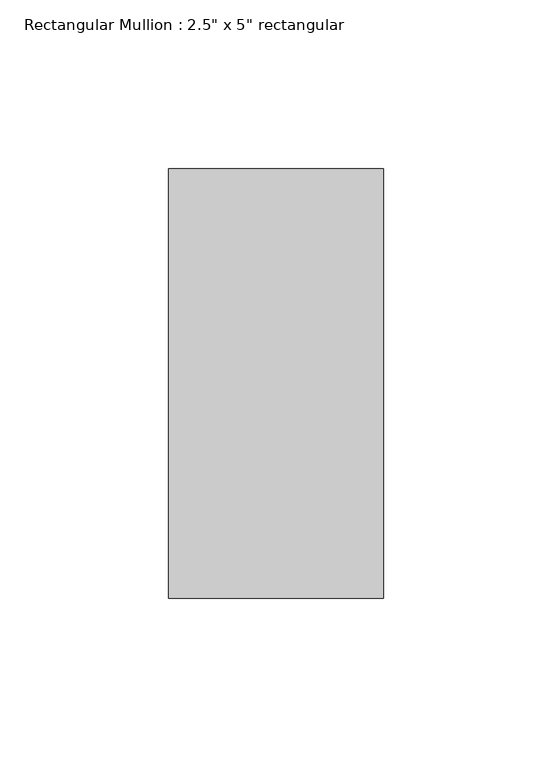
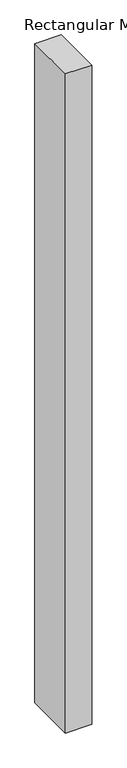
"""IFC4 building model written with IfcOpenShell, lengths in millimetres: member geometry."""

from ifc_helpers import new_model, si_unit, frame, origin, place, context, project, spatial, polyline, outline, extrude, source, transform, mapped, element, save


def member_e9b380b6(model_context):
    return source(origin(), model_context, "Body", "SweptSolid", [
        extrude(outline(polyline([(0.0, 63.5), (0.0, -63.5), (-63.5, -63.5), (-63.5, 63.5), (0.0, 63.5)])), frame((0.0, 0.0, -1678.8095798), z_axis=(0.0, 0.0, 1.0), x_axis=(1.0, 0.0, 0.0)), (0.0, 0.0, 1.0), 1678.8095798),
    ])


if __name__ == "__main__":
    model = new_model("IFC4")
    model_context = context("Model", 3, world=origin())
    ifc_project = project(units=[si_unit("LENGTHUNIT", "METRE", prefix="MILLI")], contexts=[model_context])
    site = spatial("IfcSite", under=ifc_project)
    building = spatial("IfcBuilding", under=site)
    placement = place(None, origin())
    member_shape = member_e9b380b6(model_context)
    element("IfcMember", 1, ObjectType="Rectangular Mullion : 2.5\" x 5\" rectangular", at=placement, inside=building, context=model_context, shape_type="MappedRepresentation", body=[
        mapped(member_shape, transform((0.0, 0.0, 0.0), x_axis=(1.0, 0.0, 0.0), y_axis=(0.0, 1.0, 0.0), z_axis=(0.0, 0.0, 1.0))),
    ])
    save(model, "model.ifc")

# Revit data of these elements
# Type "Rectangular Mullion : 2.5\" x 5\" rectangular"
#   built-in parameter 1007304 = 0.416667 (stored number, unit not read)
#   built-in parameter 1007301 = 0.104167 (stored number, unit not read)
#   built-in parameter 1007300 = 0.104167 (stored number, unit not read)
# Element 1 (IfcMember, "Rectangular Mullion : 2.5\" x 5\" rectangular")
#   Materials on its faces: "Aluminum"
# Materials
#   "Aluminum": class "Metal", colour RGB 247 247 247, transparency 0, Description = "Aluminum 6061", Cost = 0
